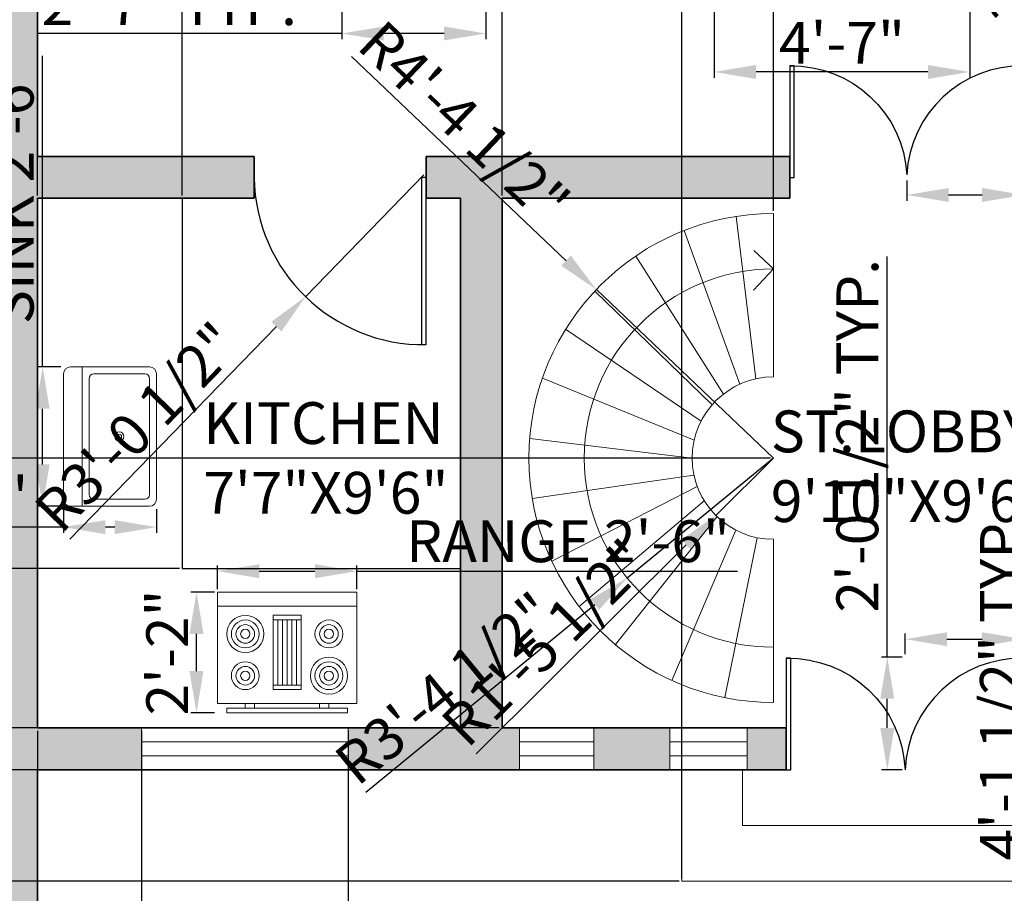
# Model space of a CAD drawing. Units: inches. Extents: x 32476 to 33108, y 58720 to 59630.
# Tile 3 of 6: x 32598 to 32810, y 58975 to 59163. Entities that reach past the tile are written whole.
import ezdxf

# ---------------------------------------------------------------- set-up
doc = ezdxf.new("R2010")
doc.units = ezdxf.units.IN
for name, color, linetype, lineweight in [('A-ANNO-DIMS', 6, 'Continuous', 18), ('A-AREA-IDEN', 32, 'Continuous', 18), ('A-DOOR', 4, 'Continuous', 25), ('A-EQPM', 9, 'Continuous', 18), ('A-FLOR-CASE', 9, 'Continuous', 25), ('A-FLOR-FIXT', 9, 'Continuous', 18), ('A-FLOR-STRS', 7, 'Continuous', 18), ('A-GLAZ', 4, 'Continuous', 18), ('A-WALL', 7, 'Continuous', 35), ('A-WALL-PATT', 251, 'Continuous', 13)]:
    doc.layers.add(name, color=color, linetype=linetype, lineweight=lineweight)
doc.styles.get("Standard").update_dxf_attribs({"font": 'arial.ttf'})
doc.dimstyles.new('ISO-25', dxfattribs={"dimtxt": 9, "dimasz": 9, "dimexe": 1.25, "dimexo": 0.625, "dimtad": 1, "dimdec": 1, "dimrnd": 9, "dimlunit": 3, "dimtxsty": 'Standard', "dimcen": 2.5, "dimadec": 0, "dimazin": 0, "dimtfac": 1, "dimtdec": 1, "dimtmove": 0, "dimatfit": 3, "dimfxl": 1, "dimarcsym": 0})

# ---------------------------------------------------------------- blocks, each defined once
blk = doc.blocks.new('Range-Oven - 30 in top')
for p, q in [((0, -3), (30, -3)), ((12, -6), (18, -6)), ((13, -20), (13, -6)), ((14, -6), (14, -20)), ((15, -20), (15, -6)), ((16, -6), (16, -20)), ((17, -20), (17, -6)), ((18, -20), (12, -20)), ((6, -24), (6, -25)), ((8, -25), (8, -24)), ((22, -25), (22, -24)), ((24, -24), (24, -25))]:
    blk.add_line(p, q)
for points in [[(0, -24), (0, 0), (30, 0), (30, -24)], [(12, -21), (12, -5), (18, -5), (18, -21)], [(2, -26), (2, -25), (28, -25), (28, -26)]]:
    blk.add_lwpolyline(points, close=True)
for centre, radius in [((6, -9), 4), ((6, -9), 3), ((24, -9), 3), ((6, -9), 2), ((6, -9), 1), ((24, -9), 2), ((24, -9), 1), ((24, -18), 4), ((6, -18), 3), ((6, -18), 2), ((24, -18), 3), ((24, -18), 2), ((6, -18), 1), ((24, -18), 1)]:
    blk.add_circle(centre, radius)
blk = doc.blocks.new('Sink-single - 30 in top')
blk.add_line((-15, -3.999996), (15, -3.999996))
for points in [[(-13.5, 0), (13.5, 0)], [(-15, -18.499996), (-15, -1.5)], [(15, -1.5), (15, -18.499996)], [(-12.5, -5.499996), (12.5, -5.499996)], [(-13.5, -17.499996), (-13.5, -6.499996)], [(13.5, -6.499996), (13.5, -17.499996)], [(12.5, -18.499996), (-12.5, -18.499996)], [(13.5, -19.999996), (-13.5, -19.999996)]]:
    blk.add_lwpolyline(points)
for radius in [1, 0.5]:
    blk.add_circle((0, -11.999996), radius)
for centre, radius, start, end in [((-13.5, -1.5), 1.5, 90, 180), ((13.5, -1.5), 1.5, 0, 90), ((-12.5, -6.499996), 1, 90, 180), ((12.5, -6.499996), 1, 0, 90), ((-13.5, -18.499996), 1.5, 180, 270), ((-12.5, -17.499996), 1, 180, 270), ((12.5, -17.499996), 1, 270, 0), ((13.5, -18.499996), 1.5, 270, 0)]:
    blk.add_arc(centre, radius, start, end)
blk = doc.blocks.new('DOOR-LOUNGE-PAIRED-LEAF')
for p, q in [((24.2, 0), (24.2, 24)), ((24.2, 24), (25.2, 24)), ((25.2, 24), (25.2, 4.5)), ((25.2, 0), (24.2, 0))]:
    blk.add_line(p, q)
blk.add_arc((24.7, -0.73), 24.73, 88.8415, 177.0325)
blk = doc.blocks.new('DOOR-PORCH-PAIRED-LEAF')
for p, q in [((24.56, 0), (24.56, 24)), ((24.56, 24), (25.56, 24)), ((25.56, 24), (25.56, 9)), ((25.56, 0), (24.56, 0))]:
    blk.add_line(p, q)
blk.add_arc((25.06, -1.08), 25.08, 88.8578, 177.5364)
blk = doc.blocks.new('*D24')
at = {"layer": 'A-ANNO-DIMS', "color": 0, "lineweight": -2, "transparency": 16777216}
for p, q in [((32815.82, 58972.53), (32815.82, 59058.97)), ((32790.33, 58972.53), (32817.07, 58972.53)), ((32815.82, 58932.18), (32815.82, 58963.53)), ((32790.33, 58923.18), (32817.07, 58923.18))]:
    blk.add_line(p, q, dxfattribs=at)
at = {"layer": 'A-ANNO-DIMS', "color": 0, "transparency": 16777216}
for points in [[(32814.32, 58963.53), (32817.32, 58963.53), (32815.82, 58972.53)], [(32814.32, 58932.18), (32817.32, 58932.18), (32815.82, 58923.18)]]:
    blk.add_solid(points, dxfattribs=at)
at = {"layer": 'Defpoints', "color": 0, "transparency": 16777216}
for p in [(32789.71, 58972.53), (32815.82, 58972.53), (32789.71, 58923.18)]:
    blk.add_point(p, dxfattribs=at)
at = {"layer": 'A-ANNO-DIMS', "color": 0, "transparency": 16777216, "insert": (32810.54, 59020.25), "char_height": 9, "attachment_point": 5, "rotation": 90}
blk.add_mtext('4\'-1 1/2" TYP.', dxfattribs=at)
blk = doc.blocks.new('*D26')
at = {"layer": 'A-ANNO-DIMS', "color": 0, "lineweight": -2, "transparency": 16777216}
for p, q in [((32667.53, 59168.57), (32667.53, 59158.95)), ((32698.53, 59168.57), (32698.53, 59158.95)), ((32667.53, 59160.2), (32602.27, 59160.2)), ((32689.53, 59160.2), (32676.53, 59160.2))]:
    blk.add_line(p, q, dxfattribs=at)
at = {"layer": 'A-ANNO-DIMS', "color": 0, "transparency": 16777216}
for points in [[(32676.53, 59161.7), (32676.53, 59158.7), (32667.53, 59160.2)], [(32689.53, 59161.7), (32689.53, 59158.7), (32698.53, 59160.2)]]:
    blk.add_solid(points, dxfattribs=at)
at = {"layer": 'Defpoints', "color": 0, "transparency": 16777216}
for p in [(32667.53, 59169.2), (32698.53, 59169.2), (32667.53, 59160.2)]:
    blk.add_point(p, dxfattribs=at)
at = {"layer": 'A-ANNO-DIMS', "color": 0, "transparency": 16777216, "insert": (32630.4, 59165.34), "char_height": 9, "attachment_point": 5}
blk.add_mtext('2\'-7" TYP.', dxfattribs=at)
blk = doc.blocks.new('*D27')
at = {"layer": 'A-ANNO-DIMS', "color": 0, "lineweight": -2, "transparency": 16777216}
for p, q in [((32789.11, 59128.59), (32789.11, 59124.19)), ((32814.31, 59128.59), (32814.31, 59124.19)), ((32798.11, 59125.44), (32805.31, 59125.44)), ((32814.31, 59125.44), (32913.96, 59125.44))]:
    blk.add_line(p, q, dxfattribs=at)
at = {"layer": 'A-ANNO-DIMS', "color": 0, "transparency": 16777216}
for points in [[(32798.11, 59126.94), (32798.11, 59123.94), (32789.11, 59125.44)], [(32805.31, 59126.94), (32805.31, 59123.94), (32814.31, 59125.44)]]:
    blk.add_solid(points, dxfattribs=at)
at = {"layer": 'Defpoints', "color": 0, "transparency": 16777216}
for p in [(32789.11, 59129.22), (32814.31, 59129.22), (32814.31, 59125.44)]:
    blk.add_point(p, dxfattribs=at)
at = {"layer": 'A-ANNO-DIMS', "color": 0, "transparency": 16777216, "insert": (32868.64, 59130.59), "char_height": 9, "attachment_point": 5}
blk.add_mtext('LEAF 2\'-1" TYP.', dxfattribs=at)
blk = doc.blocks.new('*D28')
at = {"layer": 'A-ANNO-DIMS', "color": 0, "lineweight": -2, "transparency": 16777216}
for p, q in [((32818.09, 59153.49), (32818.09, 59239.72)), ((32814.94, 59153.49), (32819.34, 59153.49)), ((32818.09, 59138.22), (32818.09, 59144.49)), ((32814.94, 59129.22), (32819.34, 59129.22))]:
    blk.add_line(p, q, dxfattribs=at)
at = {"layer": 'A-ANNO-DIMS', "color": 0, "transparency": 16777216}
for points in [[(32816.59, 59144.49), (32819.59, 59144.49), (32818.09, 59153.49)], [(32816.59, 59138.22), (32819.59, 59138.22), (32818.09, 59129.22)]]:
    blk.add_solid(points, dxfattribs=at)
at = {"layer": 'Defpoints', "color": 0, "transparency": 16777216}
for p in [(32814.31, 59153.49), (32818.09, 59153.49), (32814.31, 59129.22)]:
    blk.add_point(p, dxfattribs=at)
at = {"layer": 'A-ANNO-DIMS', "color": 0, "transparency": 16777216, "insert": (32812.81, 59201.11), "char_height": 9, "attachment_point": 5, "rotation": 90}
blk.add_mtext('2\'-0 1/2" TYP.', dxfattribs=at)
blk = doc.blocks.new('*D29')
at = {"layer": 'A-ANNO-DIMS', "color": 0, "lineweight": -2, "transparency": 16777216}
for p, q in [((32788.75, 59026.62), (32788.75, 59031.07)), ((32814.31, 59026.62), (32814.31, 59031.07)), ((32797.75, 59029.82), (32805.31, 59029.82)), ((32814.31, 59029.82), (32934.93, 59029.82))]:
    blk.add_line(p, q, dxfattribs=at)
at = {"layer": 'A-ANNO-DIMS', "color": 0, "transparency": 16777216}
for points in [[(32797.75, 59031.32), (32797.75, 59028.32), (32788.75, 59029.82)], [(32805.31, 59031.32), (32805.31, 59028.32), (32814.31, 59029.82)]]:
    blk.add_solid(points, dxfattribs=at)
at = {"layer": 'Defpoints', "color": 0, "transparency": 16777216}
for p in [(32814.31, 59029.82), (32788.75, 59025.99), (32814.31, 59025.99)]:
    blk.add_point(p, dxfattribs=at)
at = {"layer": 'A-ANNO-DIMS', "color": 0, "transparency": 16777216, "insert": (32879.12, 59035.1), "char_height": 9, "attachment_point": 5}
blk.add_mtext('LEAF 2\'-1 1/2" TYP.', dxfattribs=at)
blk = doc.blocks.new('*D30')
at = {"layer": 'A-ANNO-DIMS', "color": 0, "lineweight": -2, "transparency": 16777216}
for p, q in [((32784.92, 59025.99), (32784.92, 59112.23)), ((32788.13, 59025.99), (32783.67, 59025.99)), ((32784.92, 59010.72), (32784.92, 59016.99)), ((32788.13, 59001.72), (32783.67, 59001.72))]:
    blk.add_line(p, q, dxfattribs=at)
at = {"layer": 'A-ANNO-DIMS', "color": 0, "transparency": 16777216}
for points in [[(32783.42, 59016.99), (32786.42, 59016.99), (32784.92, 59025.99)], [(32783.42, 59010.72), (32786.42, 59010.72), (32784.92, 59001.72)]]:
    blk.add_solid(points, dxfattribs=at)
at = {"layer": 'Defpoints', "color": 0, "transparency": 16777216}
for p in [(32784.92, 59025.99), (32788.75, 59025.99), (32788.75, 59001.72)]:
    blk.add_point(p, dxfattribs=at)
at = {"layer": 'A-ANNO-DIMS', "color": 0, "transparency": 16777216, "insert": (32779.64, 59073.61), "char_height": 9, "attachment_point": 5, "rotation": 90}
blk.add_mtext('2\'-0 1/2" TYP.', dxfattribs=at)
blk = doc.blocks.new('*D32')
at = {"layer": 'A-ANNO-DIMS', "color": 0, "lineweight": -2, "transparency": 16777216}
for p, q in [((32747.67, 59164.94), (32747.67, 59150.67)), ((32802.67, 59164.94), (32802.67, 59150.67)), ((32793.67, 59151.92), (32756.67, 59151.92))]:
    blk.add_line(p, q, dxfattribs=at)
at = {"layer": 'A-ANNO-DIMS', "color": 0, "transparency": 16777216}
for points in [[(32756.67, 59153.42), (32756.67, 59150.42), (32747.67, 59151.92)], [(32793.67, 59153.42), (32793.67, 59150.42), (32802.67, 59151.92)]]:
    blk.add_solid(points, dxfattribs=at)
at = {"layer": 'Defpoints', "color": 0, "transparency": 16777216}
for p in [(32747.67, 59165.57), (32802.67, 59165.57), (32747.67, 59151.92)]:
    blk.add_point(p, dxfattribs=at)
at = {"layer": 'A-ANNO-DIMS', "color": 0, "transparency": 16777216, "insert": (32775.17, 59157.04), "char_height": 9, "attachment_point": 5}
blk.add_mtext('4\'-7"', dxfattribs=at)
blk = doc.blocks.new('*D33')
at = {"layer": 'A-ANNO-DIMS', "color": 0, "lineweight": -2, "transparency": 16777216}
for p, q in [((32640.76, 59040.59), (32640.76, 59045.71)), ((32670.76, 59040.59), (32670.76, 59045.71)), ((32649.76, 59044.46), (32661.76, 59044.46)), ((32670.76, 59044.46), (32752.68, 59044.46))]:
    blk.add_line(p, q, dxfattribs=at)
at = {"layer": 'A-ANNO-DIMS', "color": 0, "transparency": 16777216}
for points in [[(32649.76, 59045.96), (32649.76, 59042.96), (32640.76, 59044.46)], [(32661.76, 59045.96), (32661.76, 59042.96), (32670.76, 59044.46)]]:
    blk.add_solid(points, dxfattribs=at)
at = {"layer": 'Defpoints', "color": 0, "transparency": 16777216}
for p in [(32670.76, 59044.46), (32640.76, 59039.96), (32670.76, 59039.96)]:
    blk.add_point(p, dxfattribs=at)
at = {"layer": 'A-ANNO-DIMS', "color": 0, "transparency": 16777216, "insert": (32716.22, 59049.74), "char_height": 9, "attachment_point": 5}
blk.add_mtext('RANGE 2\'-6"', dxfattribs=at)
blk = doc.blocks.new('*D34')
at = {"layer": 'A-ANNO-DIMS', "color": 0, "lineweight": -2, "transparency": 16777216}
for p, q in [((32640.14, 59039.96), (32635.01, 59039.96)), ((32636.26, 59022.96), (32636.26, 59030.96)), ((32640.14, 59013.96), (32635.01, 59013.96))]:
    blk.add_line(p, q, dxfattribs=at)
at = {"layer": 'A-ANNO-DIMS', "color": 0, "transparency": 16777216}
for points in [[(32634.76, 59030.96), (32637.76, 59030.96), (32636.26, 59039.96)], [(32634.76, 59022.96), (32637.76, 59022.96), (32636.26, 59013.96)]]:
    blk.add_solid(points, dxfattribs=at)
at = {"layer": 'Defpoints', "color": 0, "transparency": 16777216}
for p in [(32636.26, 59039.96), (32640.76, 59039.96), (32640.76, 59013.96)]:
    blk.add_point(p, dxfattribs=at)
at = {"layer": 'A-ANNO-DIMS', "color": 0, "transparency": 16777216, "insert": (32631.12, 59026.96), "char_height": 9, "attachment_point": 5, "rotation": 90}
blk.add_mtext('2\'-2"', dxfattribs=at)
blk = doc.blocks.new('*D35')
at = {"layer": 'A-ANNO-DIMS', "color": 0, "lineweight": -2, "transparency": 16777216}
for p, q in [((32603.15, 59088.44), (32603.15, 59155.41)), ((32607.03, 59088.44), (32601.9, 59088.44)), ((32603.15, 59067.44), (32603.15, 59079.44)), ((32607.03, 59058.44), (32601.9, 59058.44))]:
    blk.add_line(p, q, dxfattribs=at)
at = {"layer": 'A-ANNO-DIMS', "color": 0, "transparency": 16777216}
for points in [[(32601.65, 59079.44), (32604.65, 59079.44), (32603.15, 59088.44)], [(32601.65, 59067.44), (32604.65, 59067.44), (32603.15, 59058.44)]]:
    blk.add_solid(points, dxfattribs=at)
at = {"layer": 'Defpoints', "color": 0, "transparency": 16777216}
for p in [(32603.15, 59088.44), (32607.65, 59088.44), (32607.65, 59058.44)]:
    blk.add_point(p, dxfattribs=at)
at = {"layer": 'A-ANNO-DIMS', "color": 0, "transparency": 16777216, "insert": (32597.87, 59126.43), "char_height": 9, "attachment_point": 5, "rotation": 90}
blk.add_mtext('SINK 2\'-6"', dxfattribs=at)
blk = doc.blocks.new('*D36')
at = {"layer": 'A-ANNO-DIMS', "color": 0, "lineweight": -2, "transparency": 16777216}
for p, q in [((32607.65, 59057.82), (32607.65, 59052.69)), ((32627.65, 59057.82), (32627.65, 59052.69)), ((32607.65, 59053.94), (32574.33, 59053.94)), ((32618.65, 59053.94), (32616.65, 59053.94))]:
    blk.add_line(p, q, dxfattribs=at)
at = {"layer": 'A-ANNO-DIMS', "color": 0, "transparency": 16777216}
for points in [[(32616.65, 59055.44), (32616.65, 59052.44), (32607.65, 59053.94)], [(32618.65, 59055.44), (32618.65, 59052.44), (32627.65, 59053.94)]]:
    blk.add_solid(points, dxfattribs=at)
at = {"layer": 'Defpoints', "color": 0, "transparency": 16777216}
for p in [(32607.65, 59058.44), (32627.65, 59058.44), (32607.65, 59053.94)]:
    blk.add_point(p, dxfattribs=at)
at = {"layer": 'A-ANNO-DIMS', "color": 0, "transparency": 16777216, "insert": (32586.49, 59059.16), "char_height": 9, "attachment_point": 5}
blk.add_mtext('1\'-8"', dxfattribs=at)
blk = doc.blocks.new('*D39')
at = {"layer": 'A-ANNO-DIMS', "color": 0, "lineweight": -2, "transparency": 16777216}
for p, q in [((32702.04, 59125.34), (32702.04, 59529.47)), ((32711.04, 59528.22), (32751.42, 59528.22)), ((32760.42, 59122.05), (32760.42, 59529.47))]:
    blk.add_line(p, q, dxfattribs=at)
at = {"layer": 'A-ANNO-DIMS', "color": 0, "transparency": 16777216}
for points in [[(32711.04, 59529.72), (32711.04, 59526.72), (32702.04, 59528.22)], [(32751.42, 59529.72), (32751.42, 59526.72), (32760.42, 59528.22)]]:
    blk.add_solid(points, dxfattribs=at)
at = {"layer": 'Defpoints', "color": 0, "transparency": 16777216}
for p in [(32760.42, 59528.22), (32702.04, 59124.72), (32760.42, 59121.43)]:
    blk.add_point(p, dxfattribs=at)
at = {"layer": 'A-ANNO-DIMS', "color": 0, "transparency": 16777216, "insert": (32731.23, 59533.5), "char_height": 9, "attachment_point": 5}
blk.add_mtext('4\'-10 1/2"', dxfattribs=at)
blk = doc.blocks.new('*D40')
at = {"layer": 'A-ANNO-DIMS', "color": 0, "lineweight": -2, "transparency": 16777216}
for p, q in [((32759.79, 59068.81), (32549.79, 59068.81)), ((32551.04, 59019.72), (32551.04, 59059.81)), ((32701.41, 59010.72), (32549.79, 59010.72))]:
    blk.add_line(p, q, dxfattribs=at)
at = {"layer": 'A-ANNO-DIMS', "color": 0, "transparency": 16777216}
for points in [[(32549.54, 59059.81), (32552.54, 59059.81), (32551.04, 59068.81)], [(32549.54, 59019.72), (32552.54, 59019.72), (32551.04, 59010.72)]]:
    blk.add_solid(points, dxfattribs=at)
at = {"layer": 'Defpoints', "color": 0, "transparency": 16777216}
for p in [(32551.04, 59068.81), (32760.42, 59068.81), (32702.04, 59010.72)]:
    blk.add_point(p, dxfattribs=at)
at = {"layer": 'A-ANNO-DIMS', "color": 0, "transparency": 16777216, "insert": (32545.82, 59039.76), "char_height": 9, "attachment_point": 5, "rotation": 90}
blk.add_mtext('4\'-10"', dxfattribs=at)
blk = doc.blocks.new('*D41')
at = {"layer": 'A-ANNO-DIMS', "color": 0, "lineweight": -2, "transparency": 16777216}
for p, q in [((32602.04, 59125.34), (32602.04, 59529.47)), ((32611.04, 59528.22), (32624.2, 59528.22)), ((32633.2, 59125.34), (32633.2, 59529.47))]:
    blk.add_line(p, q, dxfattribs=at)
at = {"layer": 'A-ANNO-DIMS', "color": 0, "transparency": 16777216}
for points in [[(32611.04, 59529.72), (32611.04, 59526.72), (32602.04, 59528.22)], [(32624.2, 59529.72), (32624.2, 59526.72), (32633.2, 59528.22)]]:
    blk.add_solid(points, dxfattribs=at)
at = {"layer": 'Defpoints', "color": 0, "transparency": 16777216}
for p in [(32633.2, 59528.22), (32602.04, 59124.72), (32633.2, 59124.72)]:
    blk.add_point(p, dxfattribs=at)
at = {"layer": 'A-ANNO-DIMS', "color": 0, "transparency": 16777216, "insert": (32617.62, 59533.36), "char_height": 9, "attachment_point": 5}
blk.add_mtext('2\'-7"', dxfattribs=at)
blk = doc.blocks.new('*D42')
at = {"layer": 'A-ANNO-DIMS', "color": 0, "lineweight": -2, "transparency": 16777216}
for p, q in [((32551.04, 59045.02), (32551.04, 59107.31)), ((32632.57, 59045.02), (32549.79, 59045.02)), ((32551.04, 59019.72), (32551.04, 59036.02)), ((32623.76, 59010.72), (32549.79, 59010.72))]:
    blk.add_line(p, q, dxfattribs=at)
at = {"layer": 'A-ANNO-DIMS', "color": 0, "transparency": 16777216}
for points in [[(32549.54, 59036.02), (32552.54, 59036.02), (32551.04, 59045.02)], [(32549.54, 59019.72), (32552.54, 59019.72), (32551.04, 59010.72)]]:
    blk.add_solid(points, dxfattribs=at)
at = {"layer": 'Defpoints', "color": 0, "transparency": 16777216}
for p in [(32551.04, 59045.02), (32633.2, 59045.02), (32624.39, 59010.72)]:
    blk.add_point(p, dxfattribs=at)
at = {"layer": 'A-ANNO-DIMS', "color": 0, "transparency": 16777216, "insert": (32545.76, 59080.67), "char_height": 9, "attachment_point": 5, "rotation": 90}
blk.add_mtext('2\'-10 1/2"', dxfattribs=at)
blk = doc.blocks.new('*D43')
at = {"layer": 'A-ANNO-DIMS', "color": 0, "lineweight": -2, "transparency": 16777216}
for p, q in [((32740.73, 58978.34), (32740.73, 59529.47)), ((32749.73, 59528.22), (32814.04, 59528.22)), ((32823.04, 58978.34), (32823.04, 59529.47))]:
    blk.add_line(p, q, dxfattribs=at)
at = {"layer": 'A-ANNO-DIMS', "color": 0, "transparency": 16777216}
for points in [[(32749.73, 59529.72), (32749.73, 59526.72), (32740.73, 59528.22)], [(32814.04, 59529.72), (32814.04, 59526.72), (32823.04, 59528.22)]]:
    blk.add_solid(points, dxfattribs=at)
at = {"layer": 'Defpoints', "color": 0, "transparency": 16777216}
for p in [(32823.04, 59528.22), (32740.73, 58977.72), (32823.04, 58977.72)]:
    blk.add_point(p, dxfattribs=at)
at = {"layer": 'A-ANNO-DIMS', "color": 0, "transparency": 16777216, "insert": (32781.88, 59533.5), "char_height": 9, "attachment_point": 5}
blk.add_mtext('6\'-10 1/2"', dxfattribs=at)
blk = doc.blocks.new('*D44')
at = {"layer": 'A-ANNO-DIMS', "color": 0, "lineweight": -2, "transparency": 16777216}
for p, q in [((32551.04, 59001.72), (32551.04, 59036.05)), ((32740.1, 59001.72), (32549.79, 59001.72)), ((32551.04, 58986.72), (32551.04, 58992.72)), ((32740.1, 58977.72), (32549.79, 58977.72))]:
    blk.add_line(p, q, dxfattribs=at)
at = {"layer": 'A-ANNO-DIMS', "color": 0, "transparency": 16777216}
for points in [[(32549.54, 58992.72), (32552.54, 58992.72), (32551.04, 59001.72)], [(32549.54, 58986.72), (32552.54, 58986.72), (32551.04, 58977.72)]]:
    blk.add_solid(points, dxfattribs=at)
at = {"layer": 'Defpoints', "color": 0, "transparency": 16777216}
for p in [(32551.04, 59001.72), (32740.73, 59001.72), (32740.73, 58977.72)]:
    blk.add_point(p, dxfattribs=at)
at = {"layer": 'A-ANNO-DIMS', "color": 0, "transparency": 16777216, "insert": (32545.82, 59023.38), "char_height": 9, "attachment_point": 5, "rotation": 90}
blk.add_mtext('2\'-0"', dxfattribs=at)
blk = doc.blocks.new('*D45')
at = {"layer": 'A-ANNO-DIMS', "color": 0, "lineweight": -2, "transparency": 16777216}
for p, q in [((32602.04, 59010.09), (32602.04, 58746.97)), ((32624.39, 59010.09), (32624.39, 58746.97)), ((32611.04, 58748.22), (32615.39, 58748.22)), ((32624.39, 58748.22), (32685.68, 58748.22))]:
    blk.add_line(p, q, dxfattribs=at)
at = {"layer": 'A-ANNO-DIMS', "color": 0, "transparency": 16777216}
for points in [[(32611.04, 58749.72), (32611.04, 58746.72), (32602.04, 58748.22)], [(32615.39, 58749.72), (32615.39, 58746.72), (32624.39, 58748.22)]]:
    blk.add_solid(points, dxfattribs=at)
at = {"layer": 'Defpoints', "color": 0, "transparency": 16777216}
for p in [(32602.04, 59010.72), (32624.39, 59010.72), (32624.39, 58748.22)]:
    blk.add_point(p, dxfattribs=at)
at = {"layer": 'A-ANNO-DIMS', "color": 0, "transparency": 16777216, "insert": (32659.53, 58753.5), "char_height": 9, "attachment_point": 5}
blk.add_mtext('1\'-10 1/2"', dxfattribs=at)
blk = doc.blocks.new('*D46')
at = {"layer": 'A-ANNO-DIMS', "color": 0, "lineweight": -2, "transparency": 16777216}
for p, q in [((32624.39, 59010.09), (32624.39, 58746.97)), ((32668.87, 59010.09), (32668.87, 58746.97)), ((32633.39, 58748.22), (32659.87, 58748.22)), ((32668.87, 58748.22), (32724.01, 58748.22))]:
    blk.add_line(p, q, dxfattribs=at)
at = {"layer": 'A-ANNO-DIMS', "color": 0, "transparency": 16777216}
for points in [[(32633.39, 58749.72), (32633.39, 58746.72), (32624.39, 58748.22)], [(32659.87, 58749.72), (32659.87, 58746.72), (32668.87, 58748.22)]]:
    blk.add_solid(points, dxfattribs=at)
at = {"layer": 'Defpoints', "color": 0, "transparency": 16777216}
for p in [(32624.39, 59010.72), (32668.87, 59010.72), (32668.87, 58748.22)]:
    blk.add_point(p, dxfattribs=at)
at = {"layer": 'A-ANNO-DIMS', "color": 0, "transparency": 16777216, "insert": (32700.94, 58753.5), "char_height": 9, "attachment_point": 5}
blk.add_mtext('3\'-8 1/2"', dxfattribs=at)
blk = doc.blocks.new('*D47')
at = {"layer": 'A-ANNO-DIMS', "color": 0, "lineweight": -2, "transparency": 16777216}
for p, q in [((32669.62, 59155.26), (32715.79, 59111.3)), ((32760.42, 59068.81), (32722.31, 59105.09))]:
    blk.add_line(p, q, dxfattribs=at)
at = {"layer": 'A-ANNO-DIMS', "color": 0, "transparency": 16777216}
blk.add_solid([(32716.83, 59112.38), (32714.76, 59110.21), (32722.31, 59105.09)], dxfattribs=at)
at = {"layer": 'Defpoints', "color": 0, "transparency": 16777216}
for p in [(32722.31, 59105.09), (32760.42, 59068.81)]:
    blk.add_point(p, dxfattribs=at)
at = {"layer": 'A-ANNO-DIMS', "color": 0, "transparency": 16777216, "insert": (32693.08, 59140.2), "char_height": 9, "attachment_point": 5, "rotation": 316.4057}
blk.add_mtext('R4\'-4 1/2"', dxfattribs=at)
blk = doc.blocks.new('*D48')
at = {"layer": 'A-ANNO-DIMS', "color": 0, "lineweight": -2, "transparency": 16777216}
for p, q in [((32760.42, 59068.81), (32728.93, 59042.99)), ((32672.67, 58996.87), (32721.97, 59037.29))]:
    blk.add_line(p, q, dxfattribs=at)
at = {"layer": 'A-ANNO-DIMS', "color": 0, "transparency": 16777216}
blk.add_solid([(32721.02, 59038.45), (32722.92, 59036.13), (32728.93, 59042.99)], dxfattribs=at)
at = {"layer": 'Defpoints', "color": 0, "transparency": 16777216}
for p in [(32760.42, 59068.81), (32728.93, 59042.99)]:
    blk.add_point(p, dxfattribs=at)
at = {"layer": 'A-ANNO-DIMS', "color": 0, "transparency": 16777216, "insert": (32690.49, 59018.31), "char_height": 9, "attachment_point": 5, "rotation": 39.3447}
blk.add_mtext('R3\'-4 1/2"', dxfattribs=at)
blk = doc.blocks.new('*D49')
at = {"layer": 'A-ANNO-DIMS', "color": 0, "lineweight": -2, "transparency": 16777216}
for p, q in [((32760.42, 59068.81), (32748.02, 59056.48)), ((32696.42, 59005.18), (32741.64, 59050.13))]:
    blk.add_line(p, q, dxfattribs=at)
at = {"layer": 'A-ANNO-DIMS', "color": 0, "transparency": 16777216}
blk.add_solid([(32740.58, 59051.2), (32742.69, 59049.07), (32748.02, 59056.48)], dxfattribs=at)
at = {"layer": 'Defpoints', "color": 0, "transparency": 16777216}
for p in [(32760.42, 59068.81), (32748.02, 59056.48)]:
    blk.add_point(p, dxfattribs=at)
at = {"layer": 'A-ANNO-DIMS', "color": 0, "transparency": 16777216, "insert": (32712.12, 59028.23), "char_height": 9, "attachment_point": 5, "rotation": 44.8316}
blk.add_mtext('R1\'-5 1/2"', dxfattribs=at)
blk = doc.blocks.new('*D56')
at = {"layer": 'A-ANNO-DIMS', "color": 0, "lineweight": -2, "transparency": 16777216}
for p, q in [((32685.19, 59129.76), (32659.72, 59103.55)), ((32609.01, 59051.38), (32653.45, 59097.1))]:
    blk.add_line(p, q, dxfattribs=at)
at = {"layer": 'A-ANNO-DIMS', "color": 0, "transparency": 16777216}
blk.add_solid([(32652.37, 59098.15), (32654.52, 59096.05), (32659.72, 59103.55)], dxfattribs=at)
at = {"layer": 'Defpoints', "color": 0, "transparency": 16777216}
for p in [(32685.19, 59129.76), (32659.72, 59103.55)]:
    blk.add_point(p, dxfattribs=at)
at = {"layer": 'A-ANNO-DIMS', "color": 0, "transparency": 16777216, "insert": (32624.3, 59074.69), "char_height": 9, "attachment_point": 5, "rotation": 45.8141}
blk.add_mtext('R3\'-0 1/2"', dxfattribs=at)

msp = doc.modelspace()

# ---------------------------------------------------------------- hatches: boundary and pattern name
at = {"layer": 'A-WALL-PATT'}
h = msp.add_hatch(color=256, dxfattribs=at)
h.dxf.hatch_style = 1
h.paths.add_polyline_path([(32602.04, 59418.72), (32606.39, 59418.72), (32606.39, 59423.22), (32602.04, 59423.22), (32602.04, 59477.22), (32698.04, 59477.22), (32698.04, 59469.73), (32702.54, 59469.73), (32702.54, 59481.72), (32867.54, 59481.72), (32867.54, 59427.72), (32860.2, 59427.72), (32860.2, 59418.72), (32867.54, 59418.72), (32935.14, 59418.72), (32935.14, 59423.22), (32872.04, 59423.22), (32872.04, 59477.22), (32968.04, 59477.22), (32968.04, 59423.22), (32962.36, 59423.22), (32962.36, 59418.72), (32968.04, 59418.72), (32968.04, 59286.72), (32867.54, 59286.72), (32832.04, 59286.72), (32828.7, 59289.44), (32818.99, 59279.82), (32823.04, 59277.72), (32823.04, 59269.52), (32832.04, 59269.52), (32832.04, 59277.72), (32867.54, 59277.72), (32968.04, 59277.72), (32968.04, 58880.22), (32925.88, 58880.22), (32925.88, 58871.22), (32968.04, 58871.22), (32968.04, 58799.22), (32823.04, 58799.22), (32823.04, 58790.22), (32977.04, 58790.22), (32977.04, 59486.22), (32867.54, 59486.22), (32702.54, 59486.22), (32593.04, 59486.22), (32593.04, 58803.66), (32602.04, 58803.66), (32602.04, 59001.72), (32624.39, 59001.72), (32624.39, 59010.72), (32602.04, 59010.72), (32602.04, 59124.72), (32648.65, 59124.72), (32648.65, 59133.72), (32602.04, 59133.72), (32602.04, 59277.72), (32757.41, 59277.72), (32757.41, 59279.22), (32742.07, 59288.84), (32739.6, 59286.72), (32702.54, 59286.72), (32602.04, 59286.72)])
h.paths.add_polyline_path([(32763.92, 59133.72), (32685.69, 59133.72), (32685.69, 59124.72), (32693.04, 59124.72), (32693.04, 59010.72), (32668.87, 59010.72), (32668.87, 59001.72), (32705.76, 59001.72), (32705.76, 59010.72), (32702.04, 59010.72), (32702.04, 59124.72), (32763.92, 59124.72)], flags=17)
h.paths.add_polyline_path([(32832.04, 59226.49), (32823.04, 59226.49), (32823.04, 59133.72), (32814.31, 59133.72), (32814.31, 59124.72), (32823.04, 59124.72), (32823.04, 59099.14), (32832.04, 59099.14), (32832.04, 59124.72), (32839.29, 59124.72), (32839.29, 59133.72), (32832.04, 59133.72)], flags=17)
h.paths.add_polyline_path([(32921.54, 59133.72), (32874.43, 59133.72), (32874.43, 59124.72), (32917.04, 59124.72), (32917.04, 59097.72), (32921.54, 59097.72), (32921.54, 59124.72)], flags=17)
h.paths.add_polyline_path([(32832.04, 59066.22), (32968.04, 59066.22), (32968.04, 59070.72), (32921.54, 59070.72), (32921.54, 59074.56), (32917.04, 59074.56), (32917.04, 59070.72), (32832.04, 59070.72), (32832.04, 59074.32), (32823.04, 59074.32), (32823.04, 59056.98), (32832.04, 59056.98)], flags=17)
h.paths.add_polyline_path([(32738.1, 59010.72), (32721.79, 59010.72), (32721.79, 59001.72), (32738.1, 59001.72)], flags=16)
h.paths.add_polyline_path([(32763.19, 59010.72), (32754.77, 59010.72), (32754.77, 59001.72), (32763.19, 59001.72)], flags=16)
h.paths.add_polyline_path([(32832.04, 59016.15), (32823.04, 59016.15), (32823.04, 59010.72), (32814.31, 59010.72), (32814.31, 59001.72), (32823.04, 59001.72), (32823.04, 58871.22), (32860.05, 58871.22), (32860.05, 58880.22), (32832.04, 58880.22)], flags=17)
h.paths.add_polyline_path([(32702.54, 59448.33), (32698.04, 59448.33), (32698.04, 59423.22), (32631.9, 59423.22), (32631.9, 59418.72), (32702.54, 59418.72), (32706.18, 59418.72), (32706.18, 59427.72), (32702.54, 59427.72)], flags=17)
h.paths.add_polyline_path([(32789.04, 59418.72), (32800.22, 59418.72), (32800.22, 59427.72), (32775.59, 59427.72), (32775.59, 59418.72), (32780.04, 59418.72), (32780.04, 59337.58), (32773.73, 59333.67), (32782.91, 59322.03), (32784.1, 59324.11), (32785.3, 59322.03), (32798.33, 59329.69), (32789.04, 59343.18)], flags=17)

# ---------------------------------------------------------------- linework, layer by layer
at = {"layer": 'A-DOOR'}
for p, q in [((32685.69, 59129.22), (32684.69, 59129.22)), ((32684.69, 59129.22), (32684.69, 59093.22)), ((32685.69, 59093.22), (32685.69, 59124.72)), ((32684.69, 59093.22), (32685.69, 59093.22))]:
    msp.add_line(p, q, dxfattribs=at)
msp.add_arc((32685.19, 59129.76), 36.54, 180.8437, 270.784, dxfattribs=at)
at = {"layer": 'A-FLOR-CASE'}
for p, q in [((32633.2, 59124.72), (32633.2, 59045.02)), ((32633.2, 59045.02), (32693.04, 59045.02))]:
    msp.add_line(p, q, dxfattribs=at)
at = {"layer": 'A-FLOR-STRS'}
for p, q in [((32760.42, 59121.43), (32760.42, 59086.29)), ((32756.6, 59085.87), (32752.39, 59120.81)), ((32753.22, 59084.74), (32741.18, 59117.78)), ((32760.42, 59109.52), (32756.23, 59113.46)), ((32749.65, 59082.58), (32730.78, 59112.28)), ((32760.42, 59109.52), (32756.15, 59104.98)), ((32747.2, 59080.25), (32721.98, 59104.73)), ((32744.85, 59076.76), (32715.7, 59096.53)), ((32743.36, 59072.65), (32710.69, 59086.01)), ((32742.93, 59068.81), (32707.97, 59073.01)), ((32743.32, 59065.15), (32708.53, 59060.1)), ((32744.03, 59062.72), (32712.7, 59046.63)), ((32745.54, 59059.62), (32718.6, 59036.87)), ((32747.98, 59055.82), (32726.41, 59028.66)), ((32747.98, 59055.82), (32748.33, 59056.18)), ((32752.31, 59053.32), (32738.52, 59020.96)), ((32756.95, 59051.67), (32749.97, 59017.24)), ((32760.42, 59051.32), (32760.42, 59016.19)), ((32740.73, 59001.72), (32740.73, 58977.72)), ((32753.73, 59001.72), (32753.73, 59001.72)), ((32753.73, 59001.72), (32753.73, 58989.72)), ((32753.73, 58989.72), (32823.04, 58989.72)), ((32740.73, 58977.72), (32823.04, 58977.72))]:
    msp.add_line(p, q, dxfattribs=at)
for radius in [52.62, 40.71, 17.49]:
    msp.add_arc((32760.42, 59068.81), radius, 90, 270, dxfattribs=at)
at = {"layer": 'A-GLAZ'}
for p, q in [((32624.39, 59010.72), (32624.39, 59001.72)), ((32668.87, 59010.72), (32668.87, 59001.72)), ((32705.76, 59010.72), (32705.76, 59001.72)), ((32721.79, 59010.72), (32721.79, 59001.72)), ((32738.1, 59010.72), (32738.1, 59001.72)), ((32754.77, 59010.72), (32754.77, 59001.72)), ((32668.87, 59007.72), (32624.39, 59007.72)), ((32721.79, 59007.72), (32705.76, 59007.72)), ((32754.77, 59007.72), (32738.1, 59007.72)), ((32668.87, 59004.72), (32624.39, 59004.72)), ((32721.79, 59004.72), (32705.76, 59004.72)), ((32754.77, 59004.72), (32738.1, 59004.72))]:
    msp.add_line(p, q, dxfattribs=at)
at = {"layer": 'A-WALL'}
for p, q in [((32602.04, 59277.72), (32602.04, 59133.72)), ((32648.65, 59133.72), (32602.04, 59133.72)), ((32648.65, 59133.72), (32648.65, 59124.72)), ((32685.69, 59133.72), (32685.69, 59124.72)), ((32763.92, 59133.72), (32685.69, 59133.72)), ((32763.92, 59133.72), (32763.92, 59124.72)), ((32602.04, 59124.72), (32602.04, 59010.72)), ((32648.65, 59124.72), (32602.04, 59124.72)), ((32693.04, 59124.72), (32685.69, 59124.72)), ((32693.04, 59124.72), (32693.04, 59010.72)), ((32702.04, 59124.72), (32702.04, 59010.72)), ((32763.92, 59124.72), (32702.04, 59124.72)), ((32693.04, 59010.72), (32602.04, 59010.72)), ((32763.19, 59010.72), (32702.04, 59010.72)), ((32763.19, 59010.72), (32763.19, 59001.72)), ((32763.19, 59001.72), (32602.04, 59001.72)), ((32602.04, 59001.72), (32602.04, 58803.66))]:
    msp.add_line(p, q, dxfattribs=at)

# ---------------------------------------------------------------- block references
at = {"layer": 'A-DOOR', "extrusion": (0, 0, -1), "zscale": -1}
for name, p in [('DOOR-LOUNGE-PAIRED-LEAF', (-32789.11, 59129.22)), ('DOOR-PORCH-PAIRED-LEAF', (-32788.75, 59001.72))]:
    msp.add_blockref(name, p, dxfattribs=at)
at = {"layer": 'A-DOOR'}
for name, p in [('DOOR-LOUNGE-PAIRED-LEAF', (32789.11, 59129.22)), ('DOOR-PORCH-PAIRED-LEAF', (32788.75, 59001.72))]:
    msp.add_blockref(name, p, dxfattribs=at)
at = {"layer": 'A-EQPM'}
msp.add_blockref('Range-Oven - 30 in top', (32640.76, 59039.96), dxfattribs=at)
at = {"layer": 'A-FLOR-FIXT', "rotation": 90}
msp.add_blockref('Sink-single - 30 in top', (32607.65, 59073.44), dxfattribs=at)

# ---------------------------------------------------------------- texts
at = {"layer": 'A-AREA-IDEN', "char_height": 9, "attachment_point": 1}
for s, width, insert in [('KITCHEN\\P7\'7"X9\'6"', 57.3661, (32637.72, 59080.84)), ('ST.LOBBY\\P9\'10"X9\'6"', 92.241, (32759.85, 59079.05))]:
    msp.add_mtext_dynamic_manual_height_columns(s, width=width, gutter_width=12.5, heights=[0], dxfattribs=dict(at, insert=insert))

# ---------------------------------------------------------------- dimensions: what is measured, and where the dimension line sits
at = {"layer": 'A-ANNO-DIMS'}
for base, p1, p2, picture, middle in [((32760.42, 59528.22), (32702.04, 59124.72), (32760.42, 59121.43), '*D39', (32731.23, 59533.5)), ((32823.04, 59528.22), (32740.73, 58977.72), (32823.04, 58977.72), '*D43', (32781.88, 59533.5)), ((32633.2, 59528.22), (32602.04, 59124.72), (32633.2, 59124.72), '*D41', (32617.62, 59533.36)), ((32624.3879, 58748.2191), (32602.0354, 59010.7191), (32624.3879, 59010.7191), '*D45', (32659.5334, 58753.4976)), ((32668.87, 58748.22), (32624.39, 59010.72), (32668.87, 59010.72), '*D46', (32700.94, 58753.5))]:
    dim = msp.add_linear_dim(base=base, p1=p1, p2=p2, dimstyle='ISO-25', override={"dimdec": 1, "dimlfac": 1, "dimrnd": 0, "dimzin": 1, "dimdsep": 46, "dimlunit": 4, "dimfrac": 2}, dxfattribs=at)
    dim.commit()
    dim.dimension.update_dxf_attribs({"geometry": picture, "text_midpoint": middle})
for base, p1, p2, angle, text, picture, middle in [((32818.09, 59153.49), (32814.31, 59129.22), (32814.31, 59153.49), 90, '<> TYP.', '*D28', (32812.81, 59201.11)), ((32667.53, 59160.2), (32698.53, 59169.2), (32667.53, 59169.2), 180, '<> TYP.', '*D26', (32630.4, 59165.34)), ((32603.15, 59088.44), (32607.65, 59058.44), (32607.65, 59088.44), 90, 'SINK <>', '*D35', (32597.87, 59126.43)), ((32784.92, 59025.99), (32788.75, 59001.72), (32788.75, 59025.99), 90, '<> TYP.', '*D30', (32779.64, 59073.61)), ((32815.8223, 58972.5292), (32789.7053, 58923.1843), (32789.7053, 58972.5292), 90, '<> TYP.', '*D24', (32810.5439, 59020.2507))]:
    dim = msp.add_linear_dim(base=base, p1=p1, p2=p2, angle=angle, text=text, dimstyle='ISO-25', override={"dimdec": 1, "dimlfac": 1, "dimrnd": 0, "dimzin": 1, "dimdsep": 46, "dimlunit": 4, "dimfrac": 2}, dxfattribs=at)
    dim.commit()
    dim.dimension.update_dxf_attribs({"geometry": picture, "text_midpoint": middle})
for base, p1, p2, angle, picture, middle in [((32747.67, 59151.92), (32802.67, 59165.57), (32747.67, 59165.57), 180, '*D32', (32775.17, 59157.04)), ((32551.04, 59045.02), (32624.39, 59010.72), (32633.2, 59045.02), 90, '*D42', (32545.76, 59080.67)), ((32551.04, 59068.81), (32702.04, 59010.72), (32760.42, 59068.81), 90, '*D40', (32545.82, 59039.76)), ((32607.65, 59053.94), (32627.65, 59058.44), (32607.65, 59058.44), 180, '*D36', (32586.49, 59059.16)), ((32636.26, 59039.96), (32640.76, 59013.96), (32640.76, 59039.96), 90, '*D34', (32631.12, 59026.96)), ((32551.04, 59001.72), (32740.73, 58977.72), (32740.73, 59001.72), 90, '*D44', (32545.82, 59023.38))]:
    dim = msp.add_linear_dim(base=base, p1=p1, p2=p2, angle=angle, dimstyle='ISO-25', override={"dimdec": 1, "dimlfac": 1, "dimrnd": 0, "dimzin": 1, "dimdsep": 46, "dimlunit": 4, "dimfrac": 2}, dxfattribs=at)
    dim.commit()
    dim.dimension.update_dxf_attribs({"geometry": picture, "text_midpoint": middle})
for center, mpoint, picture, middle in [((32760.42, 59068.81), (32722.31, 59105.09), '*D47', (32693.08, 59140.2)), ((32685.19, 59129.76), (32659.72, 59103.55), '*D56', (32624.3, 59074.69)), ((32760.42, 59068.81), (32728.93, 59042.99), '*D48', (32690.49, 59018.31)), ((32760.42, 59068.81), (32748.02, 59056.48), '*D49', (32712.12, 59028.23))]:
    dim = msp.add_radius_dim(center=center, mpoint=mpoint, dimstyle='ISO-25', override={"dimdec": 1, "dimlfac": 1, "dimrnd": 0, "dimzin": 1, "dimdsep": 46, "dimlunit": 4, "dimfrac": 2}, dxfattribs=at)
    dim.commit()
    dim.dimension.update_dxf_attribs({"geometry": picture, "text_midpoint": middle})
for base, p1, p2, text, picture, middle in [((32814.31, 59125.44), (32789.11, 59129.22), (32814.31, 59129.22), 'LEAF <> TYP.', '*D27', (32868.64, 59130.59)), ((32670.76, 59044.46), (32640.76, 59039.96), (32670.76, 59039.96), 'RANGE <>', '*D33', (32716.22, 59049.74)), ((32814.31, 59029.82), (32788.75, 59025.99), (32814.31, 59025.99), 'LEAF <> TYP.', '*D29', (32879.12, 59035.1))]:
    dim = msp.add_linear_dim(base=base, p1=p1, p2=p2, text=text, dimstyle='ISO-25', override={"dimdec": 1, "dimlfac": 1, "dimrnd": 0, "dimzin": 1, "dimdsep": 46, "dimlunit": 4, "dimfrac": 2}, dxfattribs=at)
    dim.commit()
    dim.dimension.update_dxf_attribs({"geometry": picture, "text_midpoint": middle})

doc.saveas('drawing.dxf')
